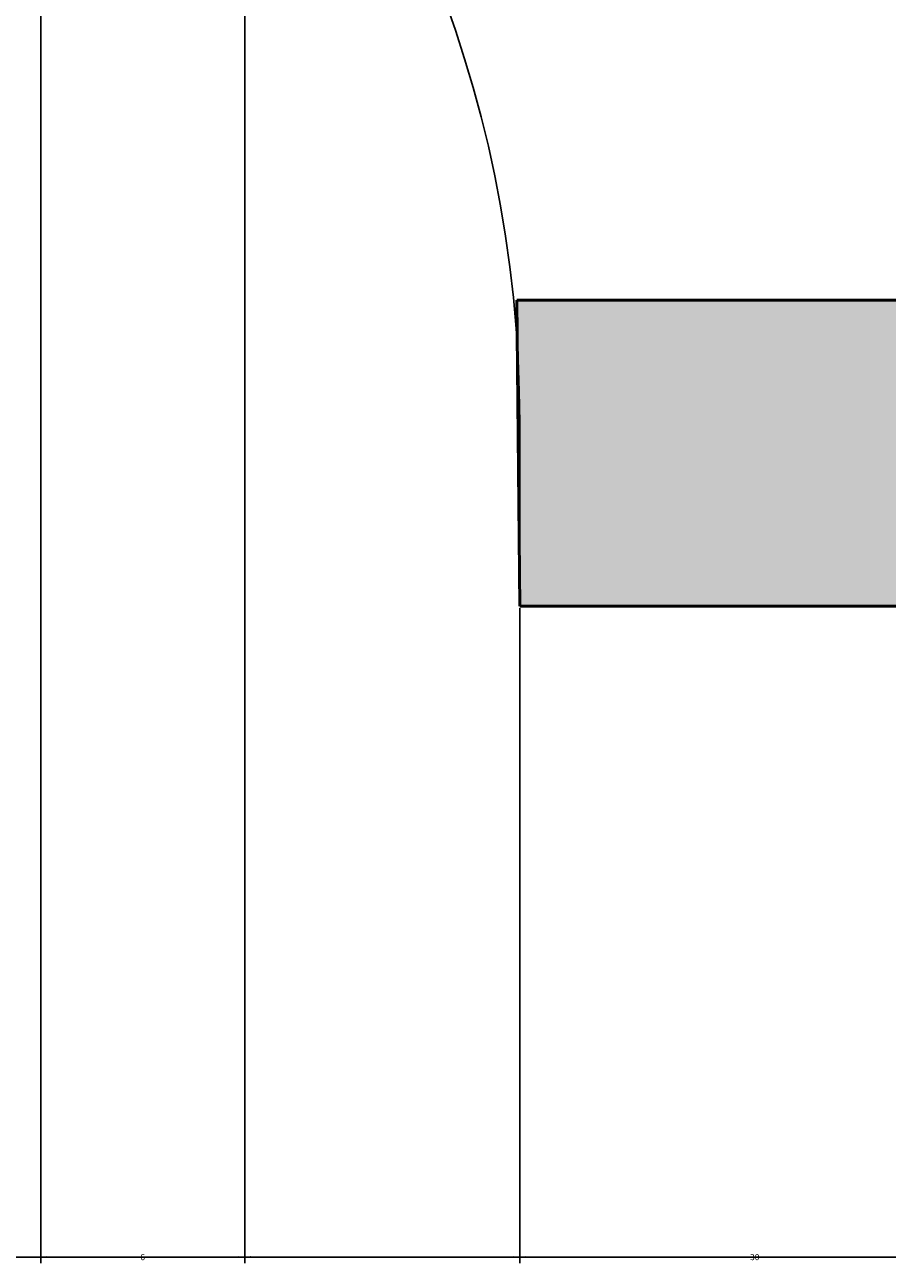
# Model space of a CAD drawing. Units: inches. Extents: x 2307 to 2544, y 2171 to 2540.
# Tile 8 of 52: x 2455 to 2481, y 2171 to 2208. Entities that reach past the tile are written whole.
import ezdxf

# ---------------------------------------------------------------- set-up
doc = ezdxf.new("R2010")
doc.units = ezdxf.units.IN
for name, color, linetype, lineweight in [('A-ANNO-DIMS', 2, 'Continuous', 18), ('A-DOOR', 3, 'Continuous', 25), ('A-WALL', 7, 'Continuous', 50)]:
    doc.layers.add(name, color=color, linetype=linetype, lineweight=lineweight)
doc.layers.add('A-WALL-PATT', color=18, linetype='Continuous', lineweight=13, true_color=0x000000)
doc.styles.get("Standard").update_dxf_attribs({"font": 'arial.ttf'})
doc.dimstyles.get("Standard").update_dxf_attribs({"dimtxt": 0.18, "dimasz": 0.18, "dimexe": 0.18, "dimexo": 0.0625, "dimgap": 0.09, "dimtad": 0, "dimtih": 1, "dimtoh": 1, "dimdec": 4, "dimzin": 0, "dimdsep": 46, "dimtxsty": 'Standard', "dimcen": 0.09, "dimadec": 0, "dimazin": 0, "dimtfac": 1, "dimtdec": 4, "dimtofl": 0, "dimtmove": 0, "dimatfit": 3, "dimfxl": 1, "dimtolj": 1, "dimtzin": 0, "dimarcsym": 0})

# ---------------------------------------------------------------- blocks, each defined once
blk = doc.blocks.new('*U13')
blk.add_line((40, 0), (40, -6))
blk.add_arc((0, 0), 40, 0, 90)
blk = doc.blocks.new('*D36')
at = {"layer": 'A-ANNO-DIMS', "color": 0, "lineweight": -2, "transparency": 16777216}
for p, q in [((2326.696, 2190.447), (2326.696, 2171.18)), ((2524.696, 2190.447), (2524.696, 2171.18)), ((2326.876, 2171.36), (2425.415, 2171.36)), ((2524.516, 2171.36), (2425.976, 2171.36))]:
    blk.add_line(p, q, dxfattribs=at)
at = {"layer": 'A-ANNO-DIMS', "color": 0, "transparency": 16777216}
for points in [[(2326.876, 2171.39), (2326.876, 2171.33), (2326.696, 2171.36)], [(2524.516, 2171.39), (2524.516, 2171.33), (2524.696, 2171.36)]]:
    blk.add_solid(points, dxfattribs=at)
at = {"layer": 'Defpoints', "color": 0, "transparency": 16777216}
for p in [(2326.696, 2190.51), (2524.696, 2190.51), (2524.696, 2171.36)]:
    blk.add_point(p, dxfattribs=at)
at = {"layer": 'A-ANNO-DIMS', "color": 0, "transparency": 16777216, "insert": (2425.696, 2171.36), "char_height": 0.18, "attachment_point": 5}
blk.add_mtext('\\A1;198', dxfattribs=at)
blk = doc.blocks.new('*D39')
at = {"layer": 'A-ANNO-DIMS', "color": 0, "lineweight": -2, "transparency": 16777216}
for p, q in [((2469.783, 2190.447), (2469.783, 2171.18)), ((2524.696, 2190.447), (2524.696, 2171.18)), ((2469.963, 2171.36), (2496.863, 2171.36)), ((2524.516, 2171.36), (2497.616, 2171.36))]:
    blk.add_line(p, q, dxfattribs=at)
at = {"layer": 'A-ANNO-DIMS', "color": 0, "transparency": 16777216}
for points in [[(2469.963, 2171.39), (2469.963, 2171.33), (2469.783, 2171.36)], [(2524.516, 2171.39), (2524.516, 2171.33), (2524.696, 2171.36)]]:
    blk.add_solid(points, dxfattribs=at)
at = {"layer": 'Defpoints', "color": 0, "transparency": 16777216}
for p in [(2469.783, 2190.51), (2524.696, 2190.51), (2524.696, 2171.36)]:
    blk.add_point(p, dxfattribs=at)
at = {"layer": 'A-ANNO-DIMS', "color": 0, "transparency": 16777216, "insert": (2497.24, 2171.36), "char_height": 0.18, "attachment_point": 5}
blk.add_mtext('\\A1;54.91', dxfattribs=at)
blk = doc.blocks.new('*D40')
at = {"layer": 'A-ANNO-DIMS', "color": 0, "lineweight": -2, "transparency": 16777216}
for p, q in [((2433.783, 2190.447), (2433.783, 2171.18)), ((2469.783, 2190.447), (2469.783, 2171.18)), ((2433.963, 2171.36), (2451.564, 2171.36)), ((2469.603, 2171.36), (2452.002, 2171.36))]:
    blk.add_line(p, q, dxfattribs=at)
at = {"layer": 'A-ANNO-DIMS', "color": 0, "transparency": 16777216}
for points in [[(2433.963, 2171.39), (2433.963, 2171.33), (2433.783, 2171.36)], [(2469.603, 2171.39), (2469.603, 2171.33), (2469.783, 2171.36)]]:
    blk.add_solid(points, dxfattribs=at)
at = {"layer": 'Defpoints', "color": 0, "transparency": 16777216}
for p in [(2433.783, 2190.51), (2469.783, 2190.51), (2469.783, 2171.36)]:
    blk.add_point(p, dxfattribs=at)
at = {"layer": 'A-ANNO-DIMS', "color": 0, "transparency": 16777216, "insert": (2451.783, 2171.36), "char_height": 0.18, "attachment_point": 5}
blk.add_mtext('\\A1;36', dxfattribs=at)
blk = doc.blocks.new('*D53')
at = {"layer": 'A-ANNO-DIMS', "color": 0, "lineweight": -2, "transparency": 16777216}
for p, q in [((2455.696, 2439.447), (2455.696, 2171.18)), ((2461.696, 2439.447), (2461.696, 2171.18)), ((2455.876, 2171.36), (2458.546, 2171.36)), ((2461.516, 2171.36), (2458.845, 2171.36))]:
    blk.add_line(p, q, dxfattribs=at)
at = {"layer": 'A-ANNO-DIMS', "color": 0, "transparency": 16777216}
for points in [[(2455.876, 2171.39), (2455.876, 2171.33), (2455.696, 2171.36)], [(2461.516, 2171.39), (2461.516, 2171.33), (2461.696, 2171.36)]]:
    blk.add_solid(points, dxfattribs=at)
at = {"layer": 'Defpoints', "color": 0, "transparency": 16777216}
for p in [(2455.696, 2439.51), (2461.696, 2439.51), (2461.696, 2171.36)]:
    blk.add_point(p, dxfattribs=at)
at = {"layer": 'A-ANNO-DIMS', "color": 0, "transparency": 16777216, "insert": (2458.696, 2171.36), "char_height": 0.18, "attachment_point": 5}
blk.add_mtext('\\A1;6', dxfattribs=at)
blk = doc.blocks.new('*D54')
at = {"layer": 'A-ANNO-DIMS', "color": 0, "lineweight": -2, "transparency": 16777216}
for p, q in [((2461.696, 2435.447), (2461.696, 2171.18)), ((2491.696, 2435.447), (2491.696, 2171.18)), ((2461.876, 2171.36), (2476.477, 2171.36)), ((2491.516, 2171.36), (2476.914, 2171.36))]:
    blk.add_line(p, q, dxfattribs=at)
at = {"layer": 'A-ANNO-DIMS', "color": 0, "transparency": 16777216}
for points in [[(2461.876, 2171.39), (2461.876, 2171.33), (2461.696, 2171.36)], [(2491.516, 2171.39), (2491.516, 2171.33), (2491.696, 2171.36)]]:
    blk.add_solid(points, dxfattribs=at)
at = {"layer": 'Defpoints', "color": 0, "transparency": 16777216}
for p in [(2461.696, 2435.51), (2491.696, 2435.51), (2491.696, 2171.36)]:
    blk.add_point(p, dxfattribs=at)
at = {"layer": 'A-ANNO-DIMS', "color": 0, "transparency": 16777216, "insert": (2476.696, 2171.36), "char_height": 0.18, "attachment_point": 5}
blk.add_mtext('\\A1;30', dxfattribs=at)

msp = doc.modelspace()

# ---------------------------------------------------------------- hatches: boundary and pattern name
at = {"layer": 'A-WALL-PATT'}
h = msp.add_hatch(color=256, dxfattribs=at)
h.dxf.hatch_style = 1
h.paths.add_polyline_path([(2433.6935, 2199.5096), (2415.6423, 2199.5096), (2415.6423, 2190.5096), (2433.7832, 2190.5096)], flags=17)
h.paths.add_polyline_path([(2367.6423, 2199.5096), (2335.6958, 2199.5096), (2335.6958, 2307.3983), (2326.6958, 2307.3983), (2326.6958, 2190.5096), (2367.6423, 2190.5096)])
h.paths.add_polyline_path([(2524.6958, 2520.5096), (2496.7832, 2520.5096), (2496.7832, 2515.5149), (2472.7832, 2515.5149), (2472.7832, 2520.5096), (2415.4028, 2520.5096), (2415.4028, 2511.5096), (2451.6958, 2511.5096), (2451.6958, 2439.5096), (2451.6958, 2391.5096), (2445.6958, 2391.5096), (2445.6958, 2387.5096), (2455.6958, 2387.5096), (2455.6958, 2435.5096), (2461.6958, 2435.5096), (2461.6958, 2439.5096), (2455.6958, 2439.5096), (2455.6958, 2511.5096), (2515.6958, 2511.5096), (2515.6958, 2439.5096), (2491.6958, 2439.5096), (2491.6958, 2435.5096), (2515.6958, 2435.5096), (2515.6958, 2319.5096), (2451.6958, 2319.5096), (2451.6958, 2281.5096), (2481.6958, 2281.5096), (2481.6958, 2225.5096), (2485.6958, 2225.5096), (2485.6958, 2285.5096), (2455.6958, 2285.5096), (2455.6958, 2315.5096), (2515.6958, 2315.5096), (2515.6958, 2199.5096), (2469.6952, 2199.5096), (2469.785, 2190.5096), (2524.6958, 2190.5096)])

# ---------------------------------------------------------------- linework, layer by layer
at = {"layer": 'A-WALL'}
for p, q in [((2515.6958, 2199.5096), (2469.6952, 2199.5096)), ((2469.6952, 2199.5096), (2469.785, 2190.5096))]:
    msp.add_line(p, q, dxfattribs=at)
msp.add_lwpolyline([(2433.7832, 2190.5096), (2326.6958, 2190.5096), (2326.6958, 2520.5096), (2524.6958, 2520.5096), (2524.6958, 2190.5096), (2469.785, 2190.5096)], dxfattribs=at)

# ---------------------------------------------------------------- block references
at = {"layer": 'A-DOOR', "xscale": 0.9, "yscale": 0.9, "zscale": 0.9}
msp.add_blockref('*U13', (2433.7832, 2195.9096), dxfattribs=at)

# ---------------------------------------------------------------- dimensions: what is measured, and where the dimension line sits
at = {"layer": 'A-ANNO-DIMS'}
for base, p1, p2, override, picture, middle in [((2461.6958, 2171.3596), (2455.6958, 2439.5096), (2461.6958, 2439.5096), {"dimdec": 0, "dimlfac": 1, "dimrnd": 0, "dimzin": 0, "dimdsep": 46, "dimlunit": 2}, '*D53', (2458.6958, 2171.3596)), ((2491.6958, 2171.3596), (2461.6958, 2435.5096), (2491.6958, 2435.5096), {"dimdec": 0, "dimlfac": 1, "dimrnd": 0, "dimzin": 0, "dimdsep": 46, "dimlunit": 2}, '*D54', (2476.6958, 2171.3596)), ((2524.6958, 2171.3596), (2326.6958, 2190.5096), (2524.6958, 2190.5096), {"dimdec": 0, "dimlfac": 1, "dimrnd": 0, "dimzin": 0, "dimdsep": 46, "dimlunit": 2}, '*D36', (2425.6958, 2171.3596)), ((2469.7832, 2171.3596), (2433.7832, 2190.5096), (2469.7832, 2190.5096), {"dimdec": 0, "dimlfac": 1, "dimrnd": 0, "dimzin": 0, "dimdsep": 46, "dimlunit": 2}, '*D40', (2451.7832, 2171.3596)), ((2524.6958, 2171.3596), (2469.7832, 2190.5096), (2524.6958, 2190.5096), {"dimdec": 2, "dimlfac": 1, "dimrnd": 0, "dimzin": 0, "dimdsep": 46, "dimlunit": 2}, '*D39', (2497.2395, 2171.3596))]:
    dim = msp.add_linear_dim(base=base, p1=p1, p2=p2, dimstyle='Standard', override=override, dxfattribs=at)
    dim.commit()
    dim.dimension.update_dxf_attribs({"geometry": picture, "text_midpoint": middle})

doc.saveas('drawing.dxf')
